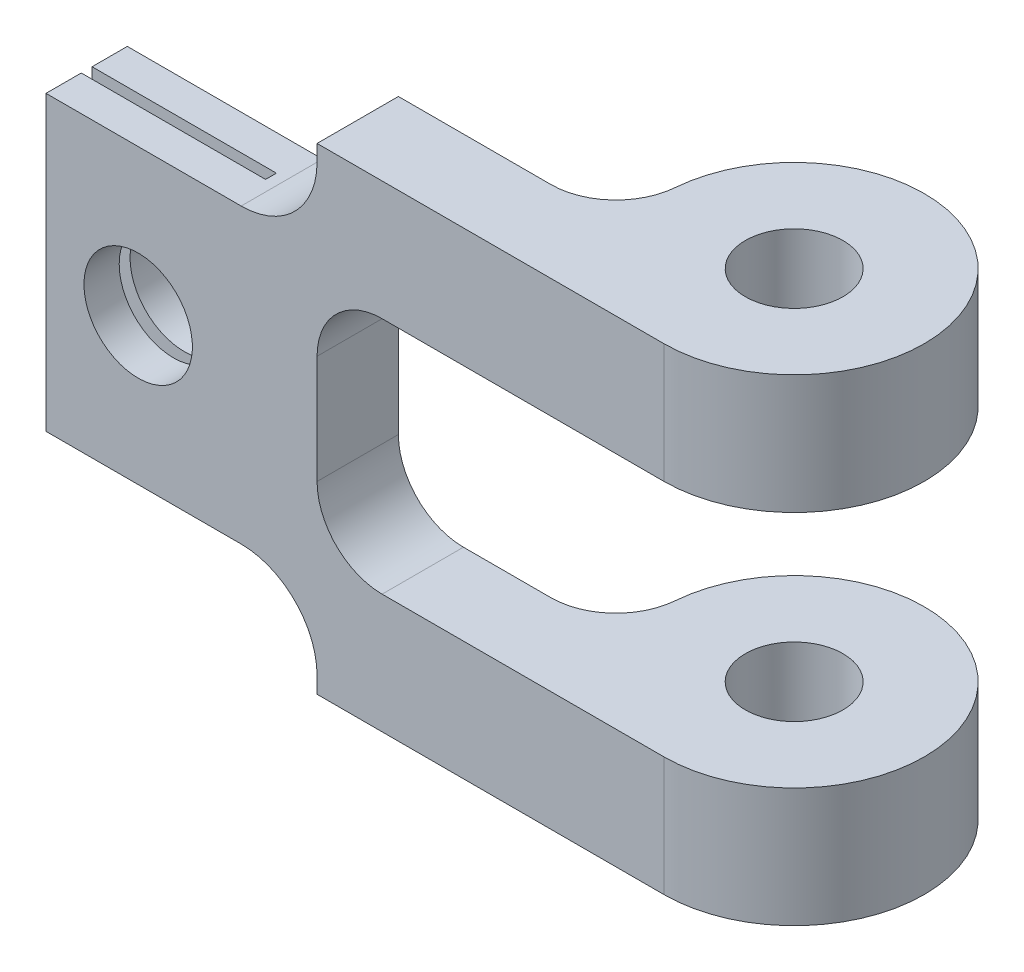
ISO-10303-21;
HEADER;
FILE_DESCRIPTION(('STEP AP214'),'2;1');
FILE_NAME('part.step','',(''),(''),'','','');
FILE_SCHEMA(('AUTOMOTIVE_DESIGN { 1 0 10303 214 1 1 1 1 }'));
ENDSEC;
DATA;
#1=APPLICATION_CONTEXT('core data for automotive mechanical design processes');
#2=APPLICATION_PROTOCOL_DEFINITION('international standard','automotive_design',2000,#1);
#3=PRODUCT_CONTEXT('',#1,'mechanical');
#4=PRODUCT('Part','Part','',(#3));
#5=PRODUCT_RELATED_PRODUCT_CATEGORY('part','',(#4));
#6=PRODUCT_DEFINITION_FORMATION('','',#4);
#7=PRODUCT_DEFINITION_CONTEXT('part definition',#1,'design');
#8=PRODUCT_DEFINITION('design','',#6,#7);
#9=PRODUCT_DEFINITION_SHAPE('','',#8);
#10=(LENGTH_UNIT() NAMED_UNIT(*) SI_UNIT(.MILLI.,.METRE.));
#11=(NAMED_UNIT(*) PLANE_ANGLE_UNIT() SI_UNIT($,.RADIAN.));
#12=(NAMED_UNIT(*) SI_UNIT($,.STERADIAN.) SOLID_ANGLE_UNIT());
#13=UNCERTAINTY_MEASURE_WITH_UNIT(LENGTH_MEASURE(1.E-05),#10,'distance_accuracy_value','');
#14=(GEOMETRIC_REPRESENTATION_CONTEXT(3) GLOBAL_UNCERTAINTY_ASSIGNED_CONTEXT((#13)) GLOBAL_UNIT_ASSIGNED_CONTEXT((#10,
#11,#12)) REPRESENTATION_CONTEXT('',''));
#15=CARTESIAN_POINT('',(0.,0.,0.));
#16=DIRECTION('',(0.,0.,1.));
#17=DIRECTION('',(1.,0.,0.));
#18=AXIS2_PLACEMENT_3D('',#15,#16,#17);
#19=CARTESIAN_POINT('',(-35.8747822293042,44.,-2.99999999999999));
#20=DIRECTION('',(0.,-1.,0.));
#21=DIRECTION('',(0.,0.,-1.));
#22=AXIS2_PLACEMENT_3D('',#19,#20,#21);
#23=CYLINDRICAL_SURFACE('',#22,12.);
#24=DIRECTION('',(0.,-1.,0.));
#25=VECTOR('',#24,1.);
#26=CARTESIAN_POINT('',(-23.9165214862028,44.,-1.99999999999999));
#27=LINE('',#26,#25);
#28=CARTESIAN_POINT('',(-23.9165214862028,44.,-1.99999999999999));
#29=VERTEX_POINT('',#28);
#30=CARTESIAN_POINT('',(-23.9165214862028,22.,-1.99999999999999));
#31=VERTEX_POINT('',#30);
#32=EDGE_CURVE('E437',#29,#31,#27,.T.);
#33=ORIENTED_EDGE('',*,*,#32,.T.);
#34=CARTESIAN_POINT('',(-35.8747822293042,22.,-2.99999999999999));
#35=DIRECTION('',(0.,1.,0.));
#36=DIRECTION('',(0.,0.,1.));
#37=AXIS2_PLACEMENT_3D('',#34,#35,#36);
#38=CIRCLE('',#37,12.);
#39=CARTESIAN_POINT('',(-35.8747822293042,22.,9.00000000000001));
#40=VERTEX_POINT('',#39);
#41=EDGE_CURVE('E290',#31,#40,#38,.F.);
#42=ORIENTED_EDGE('',*,*,#41,.T.);
#43=DIRECTION('',(0.,-1.,0.));
#44=VECTOR('',#43,1.);
#45=CARTESIAN_POINT('',(-35.8747822293042,44.,9.00000000000001));
#46=LINE('',#45,#44);
#47=CARTESIAN_POINT('',(-35.8747822293042,44.,9.00000000000001));
#48=VERTEX_POINT('',#47);
#49=EDGE_CURVE('E451',#48,#40,#46,.T.);
#50=ORIENTED_EDGE('',*,*,#49,.F.);
#51=CARTESIAN_POINT('',(-35.8747822293042,44.,-2.99999999999999));
#52=DIRECTION('',(0.,-1.,0.));
#53=DIRECTION('',(0.,0.,-1.));
#54=AXIS2_PLACEMENT_3D('',#51,#52,#53);
#55=CIRCLE('',#54,12.);
#56=EDGE_CURVE('E411',#29,#48,#55,.T.);
#57=ORIENTED_EDGE('',*,*,#56,.F.);
#58=EDGE_LOOP('',(#33,#42,#50,#57));
#59=FACE_BOUND('',#58,.T.);
#60=ADVANCED_FACE('F39',(#59),#23,.F.);
#61=CARTESIAN_POINT('',(0.,44.,0.));
#62=DIRECTION('',(0.,-1.,0.));
#63=DIRECTION('',(0.,0.,-1.));
#64=AXIS2_PLACEMENT_3D('',#61,#62,#63);
#65=CYLINDRICAL_SURFACE('',#64,24.);
#66=DIRECTION('',(0.,-1.,0.));
#67=VECTOR('',#66,1.);
#68=CARTESIAN_POINT('',(0.,44.,24.));
#69=LINE('',#68,#67);
#70=CARTESIAN_POINT('',(0.,44.,24.));
#71=VERTEX_POINT('',#70);
#72=CARTESIAN_POINT('',(0.,22.,24.));
#73=VERTEX_POINT('',#72);
#74=EDGE_CURVE('E442',#71,#73,#69,.T.);
#75=ORIENTED_EDGE('',*,*,#74,.T.);
#76=CARTESIAN_POINT('',(0.,22.,0.));
#77=DIRECTION('',(0.,1.,0.));
#78=DIRECTION('',(0.,0.,1.));
#79=AXIS2_PLACEMENT_3D('',#76,#77,#78);
#80=CIRCLE('',#79,24.);
#81=EDGE_CURVE('E284',#73,#31,#80,.T.);
#82=ORIENTED_EDGE('',*,*,#81,.T.);
#83=ORIENTED_EDGE('',*,*,#32,.F.);
#84=CARTESIAN_POINT('',(0.,44.,0.));
#85=DIRECTION('',(0.,1.,0.));
#86=DIRECTION('',(0.,0.,1.));
#87=AXIS2_PLACEMENT_3D('',#84,#85,#86);
#88=CIRCLE('',#87,24.);
#89=EDGE_CURVE('E421',#71,#29,#88,.T.);
#90=ORIENTED_EDGE('',*,*,#89,.F.);
#91=EDGE_LOOP('',(#75,#82,#83,#90));
#92=FACE_BOUND('',#91,.T.);
#93=ADVANCED_FACE('F509',(#92),#65,.T.);
#94=CARTESIAN_POINT('',(0.,44.,0.));
#95=DIRECTION('',(0.,-1.,0.));
#96=DIRECTION('',(0.,0.,-1.));
#97=AXIS2_PLACEMENT_3D('',#94,#95,#96);
#98=CYLINDRICAL_SURFACE('',#97,9.);
#99=CARTESIAN_POINT('',(0.,22.,0.));
#100=DIRECTION('',(0.,1.,0.));
#101=DIRECTION('',(0.,0.,1.));
#102=AXIS2_PLACEMENT_3D('',#99,#100,#101);
#103=CIRCLE('',#102,9.);
#104=CARTESIAN_POINT('',(0.,22.,9.));
#105=VERTEX_POINT('',#104);
#106=EDGE_CURVE('E43',#105,#105,#103,.T.);
#107=ORIENTED_EDGE('',*,*,#106,.F.);
#108=EDGE_LOOP('',(#107));
#109=FACE_BOUND('',#108,.T.);
#110=CARTESIAN_POINT('',(0.,44.,0.));
#111=DIRECTION('',(0.,1.,0.));
#112=DIRECTION('',(0.,0.,1.));
#113=AXIS2_PLACEMENT_3D('',#110,#111,#112);
#114=CIRCLE('',#113,9.);
#115=CARTESIAN_POINT('',(0.,44.,9.));
#116=VERTEX_POINT('',#115);
#117=EDGE_CURVE('E410',#116,#116,#114,.T.);
#118=ORIENTED_EDGE('',*,*,#117,.T.);
#119=EDGE_LOOP('',(#118));
#120=FACE_BOUND('',#119,.T.);
#121=ADVANCED_FACE('F486',(#109,#120),#98,.F.);
#122=CARTESIAN_POINT('',(-114.,44.001,17.5));
#123=DIRECTION('',(0.,0.,1.));
#124=DIRECTION('',(1.,0.,0.));
#125=AXIS2_PLACEMENT_3D('',#122,#123,#124);
#126=PLANE('',#125);
#127=DIRECTION('',(0.,-1.,0.));
#128=VECTOR('',#127,1.);
#129=CARTESIAN_POINT('',(-80.,44.001,17.5));
#130=LINE('',#129,#128);
#131=CARTESIAN_POINT('',(-80.,27.,17.5));
#132=VERTEX_POINT('',#131);
#133=CARTESIAN_POINT('',(-80.,20.3541019662497,17.5));
#134=VERTEX_POINT('',#133);
#135=EDGE_CURVE('E357',#132,#134,#130,.T.);
#136=ORIENTED_EDGE('',*,*,#135,.T.);
#137=DIRECTION('',(-1.,0.,0.));
#138=VECTOR('',#137,1.);
#139=CARTESIAN_POINT('',(-64.,20.3541019662497,17.5));
#140=LINE('',#139,#138);
#141=CARTESIAN_POINT('',(-114.,20.3541019662497,17.5));
#142=VERTEX_POINT('',#141);
#143=EDGE_CURVE('E329',#134,#142,#140,.T.);
#144=ORIENTED_EDGE('',*,*,#143,.T.);
#145=DIRECTION('',(0.,-1.,0.));
#146=VECTOR('',#145,1.);
#147=CARTESIAN_POINT('',(-114.,44.001,17.5));
#148=LINE('',#147,#146);
#149=CARTESIAN_POINT('',(-114.,27.,17.5));
#150=VERTEX_POINT('',#149);
#151=EDGE_CURVE('E352',#150,#142,#148,.T.);
#152=ORIENTED_EDGE('',*,*,#151,.F.);
#153=DIRECTION('',(-1.,0.,0.));
#154=VECTOR('',#153,1.);
#155=CARTESIAN_POINT('',(-114.,27.,17.5));
#156=LINE('',#155,#154);
#157=EDGE_CURVE('E343',#132,#150,#156,.T.);
#158=ORIENTED_EDGE('',*,*,#157,.F.);
#159=EDGE_LOOP('',(#136,#144,#152,#158));
#160=FACE_BOUND('',#159,.T.);
#161=ADVANCED_FACE('F605',(#160),#126,.F.);
#162=CARTESIAN_POINT('',(-97.,0.,17.5));
#163=DIRECTION('',(0.,0.,1.));
#164=DIRECTION('',(1.,0.,0.));
#165=AXIS2_PLACEMENT_3D('',#162,#163,#164);
#166=CIRCLE('',#165,9.99999999999999);
#167=CARTESIAN_POINT('',(-87.,0.,17.5));
#168=VERTEX_POINT('',#167);
#169=EDGE_CURVE('E331',#168,#168,#166,.T.);
#170=ORIENTED_EDGE('',*,*,#169,.T.);
#171=EDGE_LOOP('',(#170));
#172=FACE_BOUND('',#171,.T.);
#173=CARTESIAN_POINT('',(-114.,13.6458980337503,17.5));
#174=VERTEX_POINT('',#173);
#175=CARTESIAN_POINT('',(-114.,-13.6458980337503,17.5));
#176=VERTEX_POINT('',#175);
#177=EDGE_CURVE('E356',#174,#176,#148,.T.);
#178=ORIENTED_EDGE('',*,*,#177,.F.);
#179=DIRECTION('',(-1.,0.,0.));
#180=VECTOR('',#179,1.);
#181=CARTESIAN_POINT('',(-64.,13.6458980337503,17.5));
#182=LINE('',#181,#180);
#183=CARTESIAN_POINT('',(-80.,13.6458980337503,17.5));
#184=VERTEX_POINT('',#183);
#185=EDGE_CURVE('E322',#174,#184,#182,.F.);
#186=ORIENTED_EDGE('',*,*,#185,.T.);
#187=CARTESIAN_POINT('',(-80.,-13.6458980337503,17.5));
#188=VERTEX_POINT('',#187);
#189=EDGE_CURVE('E361',#184,#188,#130,.T.);
#190=ORIENTED_EDGE('',*,*,#189,.T.);
#191=DIRECTION('',(-1.,0.,0.));
#192=VECTOR('',#191,1.);
#193=CARTESIAN_POINT('',(-64.,-13.6458980337503,17.5));
#194=LINE('',#193,#192);
#195=EDGE_CURVE('E319',#188,#176,#194,.T.);
#196=ORIENTED_EDGE('',*,*,#195,.T.);
#197=EDGE_LOOP('',(#178,#186,#190,#196));
#198=FACE_BOUND('',#197,.T.);
#199=ADVANCED_FACE('F610',(#172,#198),#126,.F.);
#200=CARTESIAN_POINT('',(-114.,44.001,15.5));
#201=DIRECTION('',(0.,0.,-1.));
#202=DIRECTION('',(-1.,0.,0.));
#203=AXIS2_PLACEMENT_3D('',#200,#201,#202);
#204=PLANE('',#203);
#205=CARTESIAN_POINT('',(-97.,0.,15.5));
#206=DIRECTION('',(0.,0.,-1.));
#207=DIRECTION('',(-1.,0.,0.));
#208=AXIS2_PLACEMENT_3D('',#205,#206,#207);
#209=CIRCLE('',#208,9.99999999999999);
#210=CARTESIAN_POINT('',(-107.,0.,15.5));
#211=VERTEX_POINT('',#210);
#212=EDGE_CURVE('E360',#211,#211,#209,.T.);
#213=ORIENTED_EDGE('',*,*,#212,.T.);
#214=EDGE_LOOP('',(#213));
#215=FACE_BOUND('',#214,.T.);
#216=DIRECTION('',(0.,-1.,0.));
#217=VECTOR('',#216,1.);
#218=CARTESIAN_POINT('',(-80.,44.001,15.5));
#219=LINE('',#218,#217);
#220=CARTESIAN_POINT('',(-80.,13.6458980337503,15.5));
#221=VERTEX_POINT('',#220);
#222=CARTESIAN_POINT('',(-80.,-13.6458980337503,15.5));
#223=VERTEX_POINT('',#222);
#224=EDGE_CURVE('E366',#221,#223,#219,.T.);
#225=ORIENTED_EDGE('',*,*,#224,.F.);
#226=DIRECTION('',(-1.,0.,0.));
#227=VECTOR('',#226,1.);
#228=CARTESIAN_POINT('',(-64.,13.6458980337503,15.5));
#229=LINE('',#228,#227);
#230=CARTESIAN_POINT('',(-114.,13.6458980337503,15.5));
#231=VERTEX_POINT('',#230);
#232=EDGE_CURVE('E62',#221,#231,#229,.T.);
#233=ORIENTED_EDGE('',*,*,#232,.T.);
#234=DIRECTION('',(0.,-1.,0.));
#235=VECTOR('',#234,1.);
#236=CARTESIAN_POINT('',(-114.,44.001,15.5));
#237=LINE('',#236,#235);
#238=CARTESIAN_POINT('',(-114.,-13.6458980337503,15.5));
#239=VERTEX_POINT('',#238);
#240=EDGE_CURVE('E373',#231,#239,#237,.T.);
#241=ORIENTED_EDGE('',*,*,#240,.T.);
#242=DIRECTION('',(-1.,0.,0.));
#243=VECTOR('',#242,1.);
#244=CARTESIAN_POINT('',(-64.,-13.6458980337503,15.5));
#245=LINE('',#244,#243);
#246=EDGE_CURVE('E320',#239,#223,#245,.F.);
#247=ORIENTED_EDGE('',*,*,#246,.T.);
#248=EDGE_LOOP('',(#225,#233,#241,#247));
#249=FACE_BOUND('',#248,.T.);
#250=ADVANCED_FACE('F633',(#215,#249),#204,.F.);
#251=CARTESIAN_POINT('',(-80.,-20.3541019662497,15.5));
#252=VERTEX_POINT('',#251);
#253=CARTESIAN_POINT('',(-80.,-27.,15.5));
#254=VERTEX_POINT('',#253);
#255=EDGE_CURVE('E369',#252,#254,#219,.T.);
#256=ORIENTED_EDGE('',*,*,#255,.F.);
#257=DIRECTION('',(-1.,0.,0.));
#258=VECTOR('',#257,1.);
#259=CARTESIAN_POINT('',(-64.,-20.3541019662497,15.5));
#260=LINE('',#259,#258);
#261=CARTESIAN_POINT('',(-114.,-20.3541019662497,15.5));
#262=VERTEX_POINT('',#261);
#263=EDGE_CURVE('E57',#252,#262,#260,.T.);
#264=ORIENTED_EDGE('',*,*,#263,.T.);
#265=CARTESIAN_POINT('',(-114.,-27.,15.5));
#266=VERTEX_POINT('',#265);
#267=EDGE_CURVE('E351',#262,#266,#237,.T.);
#268=ORIENTED_EDGE('',*,*,#267,.T.);
#269=DIRECTION('',(1.,0.,0.));
#270=VECTOR('',#269,1.);
#271=CARTESIAN_POINT('',(-114.,-27.,15.5));
#272=LINE('',#271,#270);
#273=EDGE_CURVE('E344',#266,#254,#272,.T.);
#274=ORIENTED_EDGE('',*,*,#273,.T.);
#275=EDGE_LOOP('',(#256,#264,#268,#274));
#276=FACE_BOUND('',#275,.T.);
#277=ADVANCED_FACE('F619',(#276),#204,.F.);
#278=CARTESIAN_POINT('',(-80.,44.001,17.5));
#279=DIRECTION('',(1.,0.,0.));
#280=DIRECTION('',(0.,0.,-1.));
#281=AXIS2_PLACEMENT_3D('',#278,#279,#280);
#282=PLANE('',#281);
#283=CARTESIAN_POINT('',(-80.,27.,15.5));
#284=VERTEX_POINT('',#283);
#285=CARTESIAN_POINT('',(-80.,20.3541019662497,15.5));
#286=VERTEX_POINT('',#285);
#287=EDGE_CURVE('E364',#284,#286,#219,.T.);
#288=ORIENTED_EDGE('',*,*,#287,.T.);
#289=CARTESIAN_POINT('',(-80.,17.,16.5));
#290=DIRECTION('',(1.,0.,0.));
#291=DIRECTION('',(0.,0.,-1.));
#292=AXIS2_PLACEMENT_3D('',#289,#290,#291);
#293=CIRCLE('',#292,3.5);
#294=EDGE_CURVE('E11',#286,#134,#293,.T.);
#295=ORIENTED_EDGE('',*,*,#294,.T.);
#296=ORIENTED_EDGE('',*,*,#135,.F.);
#297=DIRECTION('',(0.,0.,1.));
#298=VECTOR('',#297,1.);
#299=CARTESIAN_POINT('',(-80.,27.,17.5));
#300=LINE('',#299,#298);
#301=EDGE_CURVE('E334',#284,#132,#300,.T.);
#302=ORIENTED_EDGE('',*,*,#301,.F.);
#303=EDGE_LOOP('',(#288,#295,#296,#302));
#304=FACE_BOUND('',#303,.T.);
#305=ADVANCED_FACE('F535',(#304),#282,.F.);
#306=ORIENTED_EDGE('',*,*,#189,.F.);
#307=EDGE_CURVE('E48',#184,#221,#293,.T.);
#308=ORIENTED_EDGE('',*,*,#307,.T.);
#309=ORIENTED_EDGE('',*,*,#224,.T.);
#310=CARTESIAN_POINT('',(-80.,-17.,16.5));
#311=DIRECTION('',(1.,0.,0.));
#312=DIRECTION('',(0.,0.,-1.));
#313=AXIS2_PLACEMENT_3D('',#310,#311,#312);
#314=CIRCLE('',#313,3.5);
#315=EDGE_CURVE('E474',#223,#188,#314,.T.);
#316=ORIENTED_EDGE('',*,*,#315,.T.);
#317=EDGE_LOOP('',(#306,#308,#309,#316));
#318=FACE_BOUND('',#317,.T.);
#319=ADVANCED_FACE('F531',(#318),#282,.F.);
#320=CARTESIAN_POINT('',(-114.,27.,97.5934779718964));
#321=DIRECTION('',(-1.,0.,0.));
#322=DIRECTION('',(0.,0.,1.));
#323=AXIS2_PLACEMENT_3D('',#320,#321,#322);
#324=PLANE('',#323);
#325=CARTESIAN_POINT('',(-114.,17.,16.5));
#326=DIRECTION('',(-1.,0.,0.));
#327=DIRECTION('',(0.,0.,1.));
#328=AXIS2_PLACEMENT_3D('',#325,#326,#327);
#329=CIRCLE('',#328,3.5);
#330=EDGE_CURVE('E308',#174,#142,#329,.T.);
#331=ORIENTED_EDGE('',*,*,#330,.F.);
#332=ORIENTED_EDGE('',*,*,#177,.T.);
#333=CARTESIAN_POINT('',(-114.,-17.,16.5));
#334=DIRECTION('',(-1.,0.,0.));
#335=DIRECTION('',(0.,0.,-1.));
#336=AXIS2_PLACEMENT_3D('',#333,#334,#335);
#337=CIRCLE('',#336,3.5);
#338=CARTESIAN_POINT('',(-114.,-20.3541019662497,17.5));
#339=VERTEX_POINT('',#338);
#340=EDGE_CURVE('E313',#339,#176,#337,.T.);
#341=ORIENTED_EDGE('',*,*,#340,.F.);
#342=CARTESIAN_POINT('',(-114.,-27.,17.5));
#343=VERTEX_POINT('',#342);
#344=EDGE_CURVE('E359',#339,#343,#148,.T.);
#345=ORIENTED_EDGE('',*,*,#344,.T.);
#346=DIRECTION('',(0.,0.,-1.));
#347=VECTOR('',#346,1.);
#348=CARTESIAN_POINT('',(-114.,-27.,97.5934779718964));
#349=LINE('',#348,#347);
#350=CARTESIAN_POINT('',(-114.,-27.,24.));
#351=VERTEX_POINT('',#350);
#352=EDGE_CURVE('E402',#351,#343,#349,.T.);
#353=ORIENTED_EDGE('',*,*,#352,.F.);
#354=DIRECTION('',(0.,-1.,0.));
#355=VECTOR('',#354,1.);
#356=CARTESIAN_POINT('',(-114.,27.,24.));
#357=LINE('',#356,#355);
#358=CARTESIAN_POINT('',(-114.,27.,24.));
#359=VERTEX_POINT('',#358);
#360=EDGE_CURVE('E383',#359,#351,#357,.T.);
#361=ORIENTED_EDGE('',*,*,#360,.F.);
#362=DIRECTION('',(0.,0.,-1.));
#363=VECTOR('',#362,1.);
#364=CARTESIAN_POINT('',(-114.,27.,97.5934779718964));
#365=LINE('',#364,#363);
#366=EDGE_CURVE('E390',#359,#150,#365,.T.);
#367=ORIENTED_EDGE('',*,*,#366,.T.);
#368=ORIENTED_EDGE('',*,*,#151,.T.);
#369=EDGE_LOOP('',(#331,#332,#341,#345,#353,#361,#367,#368));
#370=FACE_BOUND('',#369,.T.);
#371=ADVANCED_FACE('F579',(#370),#324,.T.);
#372=CARTESIAN_POINT('',(-97.,0.,24.001));
#373=DIRECTION('',(0.,0.,-1.));
#374=DIRECTION('',(-1.,0.,0.));
#375=AXIS2_PLACEMENT_3D('',#372,#373,#374);
#376=CYLINDRICAL_SURFACE('',#375,9.99999999999999);
#377=ORIENTED_EDGE('',*,*,#169,.F.);
#378=EDGE_LOOP('',(#377));
#379=FACE_BOUND('',#378,.T.);
#380=CARTESIAN_POINT('',(-97.,0.,24.));
#381=DIRECTION('',(0.,0.,-1.));
#382=DIRECTION('',(-1.,0.,0.));
#383=AXIS2_PLACEMENT_3D('',#380,#381,#382);
#384=CIRCLE('',#383,9.99999999999999);
#385=CARTESIAN_POINT('',(-107.,0.,24.));
#386=VERTEX_POINT('',#385);
#387=EDGE_CURVE('E379',#386,#386,#384,.F.);
#388=ORIENTED_EDGE('',*,*,#387,.T.);
#389=EDGE_LOOP('',(#388));
#390=FACE_BOUND('',#389,.T.);
#391=ADVANCED_FACE('F632',(#379,#390),#376,.F.);
#392=CARTESIAN_POINT('',(-64.,44.,24.));
#393=DIRECTION('',(1.,0.,0.));
#394=DIRECTION('',(0.,0.,-1.));
#395=AXIS2_PLACEMENT_3D('',#392,#393,#394);
#396=PLANE('',#395);
#397=DIRECTION('',(0.,-1.,0.));
#398=VECTOR('',#397,1.);
#399=CARTESIAN_POINT('',(-64.,44.,9.00000000000001));
#400=LINE('',#399,#398);
#401=CARTESIAN_POINT('',(-64.,44.,9.00000000000001));
#402=VERTEX_POINT('',#401);
#403=CARTESIAN_POINT('',(-64.,41.,9.00000000000001));
#404=VERTEX_POINT('',#403);
#405=EDGE_CURVE('E447',#402,#404,#400,.T.);
#406=ORIENTED_EDGE('',*,*,#405,.T.);
#407=DIRECTION('',(0.,0.,-1.));
#408=VECTOR('',#407,1.);
#409=CARTESIAN_POINT('',(-64.,41.,24.));
#410=LINE('',#409,#408);
#411=CARTESIAN_POINT('',(-64.,41.,24.));
#412=VERTEX_POINT('',#411);
#413=EDGE_CURVE('E462',#404,#412,#410,.F.);
#414=ORIENTED_EDGE('',*,*,#413,.T.);
#415=DIRECTION('',(0.,-1.,0.));
#416=VECTOR('',#415,1.);
#417=CARTESIAN_POINT('',(-64.,44.,24.));
#418=LINE('',#417,#416);
#419=CARTESIAN_POINT('',(-64.,44.,24.));
#420=VERTEX_POINT('',#419);
#421=EDGE_CURVE('E443',#420,#412,#418,.T.);
#422=ORIENTED_EDGE('',*,*,#421,.F.);
#423=DIRECTION('',(0.,0.,1.));
#424=VECTOR('',#423,1.);
#425=CARTESIAN_POINT('',(-64.,44.,24.));
#426=LINE('',#425,#424);
#427=EDGE_CURVE('E420',#402,#420,#426,.T.);
#428=ORIENTED_EDGE('',*,*,#427,.F.);
#429=EDGE_LOOP('',(#406,#414,#422,#428));
#430=FACE_BOUND('',#429,.T.);
#431=ADVANCED_FACE('F501',(#430),#396,.F.);
#432=CARTESIAN_POINT('',(-35.8747822293042,44.,-2.99999999999999));
#433=DIRECTION('',(0.,-1.,0.));
#434=DIRECTION('',(0.,0.,-1.));
#435=AXIS2_PLACEMENT_3D('',#432,#433,#434);
#436=PLANE('',#435);
#437=ORIENTED_EDGE('',*,*,#56,.T.);
#438=DIRECTION('',(-1.,0.,0.));
#439=VECTOR('',#438,1.);
#440=CARTESIAN_POINT('',(-35.8747822293042,44.,9.00000000000001));
#441=LINE('',#440,#439);
#442=EDGE_CURVE('E418',#48,#402,#441,.T.);
#443=ORIENTED_EDGE('',*,*,#442,.T.);
#444=ORIENTED_EDGE('',*,*,#427,.T.);
#445=DIRECTION('',(1.,0.,0.));
#446=VECTOR('',#445,1.);
#447=CARTESIAN_POINT('',(0.,44.,24.));
#448=LINE('',#447,#446);
#449=EDGE_CURVE('E423',#420,#71,#448,.T.);
#450=ORIENTED_EDGE('',*,*,#449,.T.);
#451=ORIENTED_EDGE('',*,*,#89,.T.);
#452=EDGE_LOOP('',(#437,#443,#444,#450,#451));
#453=FACE_BOUND('',#452,.T.);
#454=ORIENTED_EDGE('',*,*,#117,.F.);
#455=EDGE_LOOP('',(#454));
#456=FACE_BOUND('',#455,.T.);
#457=ADVANCED_FACE('F495',(#453,#456),#436,.F.);
#458=CARTESIAN_POINT('',(-35.8747822293042,-44.,-2.99999999999999));
#459=DIRECTION('',(0.,-1.,0.));
#460=DIRECTION('',(0.,0.,-1.));
#461=AXIS2_PLACEMENT_3D('',#458,#459,#460);
#462=PLANE('',#461);
#463=CARTESIAN_POINT('',(-35.8747822293042,-44.,-2.99999999999999));
#464=DIRECTION('',(0.,-1.,0.));
#465=DIRECTION('',(0.,0.,-1.));
#466=AXIS2_PLACEMENT_3D('',#463,#464,#465);
#467=CIRCLE('',#466,12.);
#468=CARTESIAN_POINT('',(-23.9165214862028,-44.,-1.99999999999999));
#469=VERTEX_POINT('',#468);
#470=CARTESIAN_POINT('',(-35.8747822293042,-44.,9.00000000000001));
#471=VERTEX_POINT('',#470);
#472=EDGE_CURVE('E409',#469,#471,#467,.T.);
#473=ORIENTED_EDGE('',*,*,#472,.F.);
#474=CARTESIAN_POINT('',(0.,-44.,0.));
#475=DIRECTION('',(0.,1.,0.));
#476=DIRECTION('',(0.,0.,1.));
#477=AXIS2_PLACEMENT_3D('',#474,#475,#476);
#478=CIRCLE('',#477,24.);
#479=CARTESIAN_POINT('',(0.,-44.,24.));
#480=VERTEX_POINT('',#479);
#481=EDGE_CURVE('E417',#480,#469,#478,.T.);
#482=ORIENTED_EDGE('',*,*,#481,.F.);
#483=DIRECTION('',(1.,0.,0.));
#484=VECTOR('',#483,1.);
#485=CARTESIAN_POINT('',(0.,-44.,24.));
#486=LINE('',#485,#484);
#487=CARTESIAN_POINT('',(-64.,-44.,24.));
#488=VERTEX_POINT('',#487);
#489=EDGE_CURVE('E432',#488,#480,#486,.T.);
#490=ORIENTED_EDGE('',*,*,#489,.F.);
#491=DIRECTION('',(0.,0.,1.));
#492=VECTOR('',#491,1.);
#493=CARTESIAN_POINT('',(-64.,-44.,24.));
#494=LINE('',#493,#492);
#495=CARTESIAN_POINT('',(-64.,-44.,9.00000000000001));
#496=VERTEX_POINT('',#495);
#497=EDGE_CURVE('E431',#496,#488,#494,.T.);
#498=ORIENTED_EDGE('',*,*,#497,.F.);
#499=DIRECTION('',(-1.,0.,0.));
#500=VECTOR('',#499,1.);
#501=CARTESIAN_POINT('',(-35.8747822293042,-44.,9.00000000000001));
#502=LINE('',#501,#500);
#503=EDGE_CURVE('E428',#471,#496,#502,.T.);
#504=ORIENTED_EDGE('',*,*,#503,.F.);
#505=EDGE_LOOP('',(#473,#482,#490,#498,#504));
#506=FACE_BOUND('',#505,.T.);
#507=CARTESIAN_POINT('',(0.,-44.,0.));
#508=DIRECTION('',(0.,1.,0.));
#509=DIRECTION('',(0.,0.,1.));
#510=AXIS2_PLACEMENT_3D('',#507,#508,#509);
#511=CIRCLE('',#510,9.);
#512=CARTESIAN_POINT('',(0.,-44.,9.));
#513=VERTEX_POINT('',#512);
#514=EDGE_CURVE('E408',#513,#513,#511,.T.);
#515=ORIENTED_EDGE('',*,*,#514,.T.);
#516=EDGE_LOOP('',(#515));
#517=FACE_BOUND('',#516,.T.);
#518=ADVANCED_FACE('F487',(#506,#517),#462,.T.);
#519=CARTESIAN_POINT('',(-35.8747822293042,-22.,9.00000000000001));
#520=VERTEX_POINT('',#519);
#521=EDGE_CURVE('E455',#520,#471,#46,.T.);
#522=ORIENTED_EDGE('',*,*,#521,.F.);
#523=CARTESIAN_POINT('',(-35.8747822293042,-22.,-2.99999999999999));
#524=DIRECTION('',(0.,-1.,0.));
#525=DIRECTION('',(0.,0.,-1.));
#526=AXIS2_PLACEMENT_3D('',#523,#524,#525);
#527=CIRCLE('',#526,12.);
#528=CARTESIAN_POINT('',(-23.9165214862028,-22.,-1.99999999999999));
#529=VERTEX_POINT('',#528);
#530=EDGE_CURVE('E283',#520,#529,#527,.F.);
#531=ORIENTED_EDGE('',*,*,#530,.T.);
#532=EDGE_CURVE('E422',#529,#469,#27,.T.);
#533=ORIENTED_EDGE('',*,*,#532,.T.);
#534=ORIENTED_EDGE('',*,*,#472,.T.);
#535=EDGE_LOOP('',(#522,#531,#533,#534));
#536=FACE_BOUND('',#535,.T.);
#537=ADVANCED_FACE('F491',(#536),#23,.F.);
#538=CARTESIAN_POINT('',(-35.8747822293042,44.,9.00000000000001));
#539=DIRECTION('',(0.,0.,1.));
#540=DIRECTION('',(1.,0.,0.));
#541=AXIS2_PLACEMENT_3D('',#538,#539,#540);
#542=PLANE('',#541);
#543=CARTESIAN_POINT('',(-97.,0.,9.00000000000001));
#544=DIRECTION('',(0.,0.,-1.));
#545=DIRECTION('',(-1.,0.,0.));
#546=AXIS2_PLACEMENT_3D('',#543,#544,#545);
#547=CIRCLE('',#546,9.99999999999999);
#548=CARTESIAN_POINT('',(-107.,0.,9.00000000000001));
#549=VERTEX_POINT('',#548);
#550=EDGE_CURVE('E340',#549,#549,#547,.T.);
#551=ORIENTED_EDGE('',*,*,#550,.F.);
#552=EDGE_LOOP('',(#551));
#553=FACE_BOUND('',#552,.T.);
#554=ORIENTED_EDGE('',*,*,#49,.T.);
#555=DIRECTION('',(-1.,0.,0.));
#556=VECTOR('',#555,1.);
#557=CARTESIAN_POINT('',(-35.8747822293042,22.,9.00000000000001));
#558=LINE('',#557,#556);
#559=CARTESIAN_POINT('',(-51.9999999999999,22.,9.00000000000001));
#560=VERTEX_POINT('',#559);
#561=EDGE_CURVE('E287',#40,#560,#558,.T.);
#562=ORIENTED_EDGE('',*,*,#561,.T.);
#563=CARTESIAN_POINT('',(-52.,10.,9.00000000000001));
#564=DIRECTION('',(0.,0.,1.));
#565=DIRECTION('',(1.,0.,0.));
#566=AXIS2_PLACEMENT_3D('',#563,#564,#565);
#567=CIRCLE('',#566,12.);
#568=CARTESIAN_POINT('',(-64.,9.99999999999992,9.00000000000001));
#569=VERTEX_POINT('',#568);
#570=EDGE_CURVE('E296',#560,#569,#567,.T.);
#571=ORIENTED_EDGE('',*,*,#570,.T.);
#572=DIRECTION('',(0.,-1.,0.));
#573=VECTOR('',#572,1.);
#574=CARTESIAN_POINT('',(-64.,44.,9.00000000000001));
#575=LINE('',#574,#573);
#576=CARTESIAN_POINT('',(-64.,-9.99999999999991,9.00000000000001));
#577=VERTEX_POINT('',#576);
#578=EDGE_CURVE('E293',#569,#577,#575,.T.);
#579=ORIENTED_EDGE('',*,*,#578,.T.);
#580=CARTESIAN_POINT('',(-52.,-10.,9.00000000000001));
#581=DIRECTION('',(0.,0.,1.));
#582=DIRECTION('',(1.,0.,0.));
#583=AXIS2_PLACEMENT_3D('',#580,#581,#582);
#584=CIRCLE('',#583,12.);
#585=CARTESIAN_POINT('',(-51.9999999999999,-22.,9.00000000000001));
#586=VERTEX_POINT('',#585);
#587=EDGE_CURVE('E291',#577,#586,#584,.T.);
#588=ORIENTED_EDGE('',*,*,#587,.T.);
#589=DIRECTION('',(1.,0.,0.));
#590=VECTOR('',#589,1.);
#591=CARTESIAN_POINT('',(-35.8747822293042,-22.,9.00000000000001));
#592=LINE('',#591,#590);
#593=EDGE_CURVE('E244',#586,#520,#592,.T.);
#594=ORIENTED_EDGE('',*,*,#593,.T.);
#595=ORIENTED_EDGE('',*,*,#521,.T.);
#596=ORIENTED_EDGE('',*,*,#503,.T.);
#597=CARTESIAN_POINT('',(-64.,-41.,9.00000000000001));
#598=VERTEX_POINT('',#597);
#599=EDGE_CURVE('E446',#598,#496,#400,.T.);
#600=ORIENTED_EDGE('',*,*,#599,.F.);
#601=CARTESIAN_POINT('',(-78.,-41.,9.00000000000001));
#602=DIRECTION('',(0.,0.,1.));
#603=DIRECTION('',(1.,0.,0.));
#604=AXIS2_PLACEMENT_3D('',#601,#602,#603);
#605=CIRCLE('',#604,14.);
#606=CARTESIAN_POINT('',(-78.,-27.,9.00000000000001));
#607=VERTEX_POINT('',#606);
#608=EDGE_CURVE('E468',#598,#607,#605,.T.);
#609=ORIENTED_EDGE('',*,*,#608,.T.);
#610=DIRECTION('',(-1.,0.,0.));
#611=VECTOR('',#610,1.);
#612=CARTESIAN_POINT('',(-64.,-27.,9.00000000000001));
#613=LINE('',#612,#611);
#614=CARTESIAN_POINT('',(-114.,-27.,9.00000000000001));
#615=VERTEX_POINT('',#614);
#616=EDGE_CURVE('E382',#607,#615,#613,.T.);
#617=ORIENTED_EDGE('',*,*,#616,.T.);
#618=DIRECTION('',(0.,1.,0.));
#619=VECTOR('',#618,1.);
#620=CARTESIAN_POINT('',(-114.,27.,9.00000000000001));
#621=LINE('',#620,#619);
#622=CARTESIAN_POINT('',(-114.,27.,9.00000000000001));
#623=VERTEX_POINT('',#622);
#624=EDGE_CURVE('E393',#615,#623,#621,.T.);
#625=ORIENTED_EDGE('',*,*,#624,.T.);
#626=DIRECTION('',(1.,0.,0.));
#627=VECTOR('',#626,1.);
#628=CARTESIAN_POINT('',(-64.,27.,9.00000000000001));
#629=LINE('',#628,#627);
#630=CARTESIAN_POINT('',(-78.,27.,9.00000000000001));
#631=VERTEX_POINT('',#630);
#632=EDGE_CURVE('E392',#623,#631,#629,.T.);
#633=ORIENTED_EDGE('',*,*,#632,.T.);
#634=CARTESIAN_POINT('',(-78.,41.,9.00000000000001));
#635=DIRECTION('',(0.,0.,1.));
#636=DIRECTION('',(1.,0.,0.));
#637=AXIS2_PLACEMENT_3D('',#634,#635,#636);
#638=CIRCLE('',#637,14.);
#639=EDGE_CURVE('E467',#631,#404,#638,.T.);
#640=ORIENTED_EDGE('',*,*,#639,.T.);
#641=ORIENTED_EDGE('',*,*,#405,.F.);
#642=ORIENTED_EDGE('',*,*,#442,.F.);
#643=EDGE_LOOP('',(#554,#562,#571,#579,#588,#594,#595,#596,#600,#609,#617,#625,#633,#640,#641,#642));
#644=FACE_BOUND('',#643,.T.);
#645=ADVANCED_FACE('F498',(#553,#644),#542,.F.);
#646=CARTESIAN_POINT('',(-64.,-41.,24.));
#647=VERTEX_POINT('',#646);
#648=EDGE_CURVE('E441',#647,#488,#418,.T.);
#649=ORIENTED_EDGE('',*,*,#648,.F.);
#650=DIRECTION('',(0.,0.,-1.));
#651=VECTOR('',#650,1.);
#652=CARTESIAN_POINT('',(-64.,-41.,24.));
#653=LINE('',#652,#651);
#654=EDGE_CURVE('E457',#647,#598,#653,.T.);
#655=ORIENTED_EDGE('',*,*,#654,.T.);
#656=ORIENTED_EDGE('',*,*,#599,.T.);
#657=ORIENTED_EDGE('',*,*,#497,.T.);
#658=EDGE_LOOP('',(#649,#655,#656,#657));
#659=FACE_BOUND('',#658,.T.);
#660=ADVANCED_FACE('F539',(#659),#396,.F.);
#661=CARTESIAN_POINT('',(0.,44.,24.));
#662=DIRECTION('',(0.,0.,-1.));
#663=DIRECTION('',(-1.,0.,0.));
#664=AXIS2_PLACEMENT_3D('',#661,#662,#663);
#665=PLANE('',#664);
#666=ORIENTED_EDGE('',*,*,#387,.F.);
#667=EDGE_LOOP('',(#666));
#668=FACE_BOUND('',#667,.T.);
#669=CARTESIAN_POINT('',(-52.,10.,24.));
#670=DIRECTION('',(0.,0.,-1.));
#671=DIRECTION('',(1.,0.,0.));
#672=AXIS2_PLACEMENT_3D('',#669,#670,#671);
#673=CIRCLE('',#672,12.);
#674=CARTESIAN_POINT('',(-64.,9.99999999999992,24.));
#675=VERTEX_POINT('',#674);
#676=CARTESIAN_POINT('',(-51.9999999999999,22.,24.));
#677=VERTEX_POINT('',#676);
#678=EDGE_CURVE('E270',#675,#677,#673,.T.);
#679=ORIENTED_EDGE('',*,*,#678,.T.);
#680=DIRECTION('',(1.,0.,0.));
#681=VECTOR('',#680,1.);
#682=CARTESIAN_POINT('',(24.,22.,24.));
#683=LINE('',#682,#681);
#684=EDGE_CURVE('E249',#677,#73,#683,.T.);
#685=ORIENTED_EDGE('',*,*,#684,.T.);
#686=ORIENTED_EDGE('',*,*,#74,.F.);
#687=ORIENTED_EDGE('',*,*,#449,.F.);
#688=ORIENTED_EDGE('',*,*,#421,.T.);
#689=CARTESIAN_POINT('',(-78.,41.,24.));
#690=DIRECTION('',(0.,0.,-1.));
#691=DIRECTION('',(-1.,0.,0.));
#692=AXIS2_PLACEMENT_3D('',#689,#690,#691);
#693=CIRCLE('',#692,14.);
#694=CARTESIAN_POINT('',(-78.,27.,24.));
#695=VERTEX_POINT('',#694);
#696=EDGE_CURVE('E472',#412,#695,#693,.T.);
#697=ORIENTED_EDGE('',*,*,#696,.T.);
#698=DIRECTION('',(-1.,0.,0.));
#699=VECTOR('',#698,1.);
#700=CARTESIAN_POINT('',(-64.,27.,24.));
#701=LINE('',#700,#699);
#702=EDGE_CURVE('E387',#695,#359,#701,.T.);
#703=ORIENTED_EDGE('',*,*,#702,.T.);
#704=ORIENTED_EDGE('',*,*,#360,.T.);
#705=DIRECTION('',(1.,0.,0.));
#706=VECTOR('',#705,1.);
#707=CARTESIAN_POINT('',(-64.,-27.,24.));
#708=LINE('',#707,#706);
#709=CARTESIAN_POINT('',(-78.,-27.,24.));
#710=VERTEX_POINT('',#709);
#711=EDGE_CURVE('E386',#351,#710,#708,.T.);
#712=ORIENTED_EDGE('',*,*,#711,.T.);
#713=CARTESIAN_POINT('',(-78.,-41.,24.));
#714=DIRECTION('',(0.,0.,-1.));
#715=DIRECTION('',(-1.,0.,0.));
#716=AXIS2_PLACEMENT_3D('',#713,#714,#715);
#717=CIRCLE('',#716,14.);
#718=EDGE_CURVE('E466',#710,#647,#717,.T.);
#719=ORIENTED_EDGE('',*,*,#718,.T.);
#720=ORIENTED_EDGE('',*,*,#648,.T.);
#721=ORIENTED_EDGE('',*,*,#489,.T.);
#722=CARTESIAN_POINT('',(0.,-22.,24.));
#723=VERTEX_POINT('',#722);
#724=EDGE_CURVE('E263',#723,#480,#69,.T.);
#725=ORIENTED_EDGE('',*,*,#724,.F.);
#726=DIRECTION('',(-1.,0.,0.));
#727=VECTOR('',#726,1.);
#728=CARTESIAN_POINT('',(24.,-22.,24.));
#729=LINE('',#728,#727);
#730=CARTESIAN_POINT('',(-51.9999999999999,-22.,24.));
#731=VERTEX_POINT('',#730);
#732=EDGE_CURVE('E245',#723,#731,#729,.T.);
#733=ORIENTED_EDGE('',*,*,#732,.T.);
#734=CARTESIAN_POINT('',(-52.,-10.,24.));
#735=DIRECTION('',(0.,0.,-1.));
#736=DIRECTION('',(-1.,0.,0.));
#737=AXIS2_PLACEMENT_3D('',#734,#735,#736);
#738=CIRCLE('',#737,12.);
#739=CARTESIAN_POINT('',(-64.,-9.99999999999991,24.));
#740=VERTEX_POINT('',#739);
#741=EDGE_CURVE('E252',#731,#740,#738,.T.);
#742=ORIENTED_EDGE('',*,*,#741,.T.);
#743=DIRECTION('',(0.,1.,0.));
#744=VECTOR('',#743,1.);
#745=CARTESIAN_POINT('',(-64.,9.99999999999991,24.));
#746=LINE('',#745,#744);
#747=EDGE_CURVE('E256',#740,#675,#746,.T.);
#748=ORIENTED_EDGE('',*,*,#747,.T.);
#749=EDGE_LOOP('',(#679,#685,#686,#687,#688,#697,#703,#704,#712,#719,#720,#721,#725,#733,#742,#748));
#750=FACE_BOUND('',#749,.T.);
#751=ADVANCED_FACE('F261',(#668,#750),#665,.F.);
#752=CARTESIAN_POINT('',(0.,-22.,0.));
#753=DIRECTION('',(0.,-1.,0.));
#754=DIRECTION('',(0.,0.,-1.));
#755=AXIS2_PLACEMENT_3D('',#752,#753,#754);
#756=CIRCLE('',#755,24.);
#757=EDGE_CURVE('E276',#529,#723,#756,.T.);
#758=ORIENTED_EDGE('',*,*,#757,.T.);
#759=ORIENTED_EDGE('',*,*,#724,.T.);
#760=ORIENTED_EDGE('',*,*,#481,.T.);
#761=ORIENTED_EDGE('',*,*,#532,.F.);
#762=EDGE_LOOP('',(#758,#759,#760,#761));
#763=FACE_BOUND('',#762,.T.);
#764=ADVANCED_FACE('F482',(#763),#65,.T.);
#765=CARTESIAN_POINT('',(0.,-22.,0.));
#766=DIRECTION('',(0.,-1.,0.));
#767=DIRECTION('',(0.,0.,-1.));
#768=AXIS2_PLACEMENT_3D('',#765,#766,#767);
#769=CIRCLE('',#768,9.);
#770=CARTESIAN_POINT('',(0.,-22.,-9.));
#771=VERTEX_POINT('',#770);
#772=EDGE_CURVE('E273',#771,#771,#769,.T.);
#773=ORIENTED_EDGE('',*,*,#772,.F.);
#774=EDGE_LOOP('',(#773));
#775=FACE_BOUND('',#774,.T.);
#776=ORIENTED_EDGE('',*,*,#514,.F.);
#777=EDGE_LOOP('',(#776));
#778=FACE_BOUND('',#777,.T.);
#779=ADVANCED_FACE('F477',(#775,#778),#98,.F.);
#780=CARTESIAN_POINT('',(-64.,27.,97.5934779718964));
#781=DIRECTION('',(0.,1.,0.));
#782=DIRECTION('',(0.,0.,1.));
#783=AXIS2_PLACEMENT_3D('',#780,#781,#782);
#784=PLANE('',#783);
#785=ORIENTED_EDGE('',*,*,#702,.F.);
#786=DIRECTION('',(0.,0.,-1.));
#787=VECTOR('',#786,1.);
#788=CARTESIAN_POINT('',(-78.,27.,97.5934779718964));
#789=LINE('',#788,#787);
#790=EDGE_CURVE('E463',#695,#631,#789,.T.);
#791=ORIENTED_EDGE('',*,*,#790,.T.);
#792=ORIENTED_EDGE('',*,*,#632,.F.);
#793=CARTESIAN_POINT('',(-114.,27.,15.5));
#794=VERTEX_POINT('',#793);
#795=EDGE_CURVE('E397',#794,#623,#365,.T.);
#796=ORIENTED_EDGE('',*,*,#795,.F.);
#797=DIRECTION('',(1.,0.,0.));
#798=VECTOR('',#797,1.);
#799=CARTESIAN_POINT('',(-114.,27.,15.5));
#800=LINE('',#799,#798);
#801=EDGE_CURVE('E336',#794,#284,#800,.T.);
#802=ORIENTED_EDGE('',*,*,#801,.T.);
#803=ORIENTED_EDGE('',*,*,#301,.T.);
#804=ORIENTED_EDGE('',*,*,#157,.T.);
#805=ORIENTED_EDGE('',*,*,#366,.F.);
#806=EDGE_LOOP('',(#785,#791,#792,#796,#802,#803,#804,#805));
#807=FACE_BOUND('',#806,.T.);
#808=ADVANCED_FACE('F483',(#807),#784,.T.);
#809=CARTESIAN_POINT('',(-114.,20.3541019662497,15.5));
#810=VERTEX_POINT('',#809);
#811=EDGE_CURVE('E302',#810,#231,#329,.T.);
#812=ORIENTED_EDGE('',*,*,#811,.F.);
#813=EDGE_CURVE('E367',#794,#810,#237,.T.);
#814=ORIENTED_EDGE('',*,*,#813,.F.);
#815=ORIENTED_EDGE('',*,*,#795,.T.);
#816=ORIENTED_EDGE('',*,*,#624,.F.);
#817=EDGE_CURVE('E400',#266,#615,#349,.T.);
#818=ORIENTED_EDGE('',*,*,#817,.F.);
#819=ORIENTED_EDGE('',*,*,#267,.F.);
#820=EDGE_CURVE('E303',#239,#262,#337,.T.);
#821=ORIENTED_EDGE('',*,*,#820,.F.);
#822=ORIENTED_EDGE('',*,*,#240,.F.);
#823=EDGE_LOOP('',(#812,#814,#815,#816,#818,#819,#821,#822));
#824=FACE_BOUND('',#823,.T.);
#825=ADVANCED_FACE('F594',(#824),#324,.T.);
#826=CARTESIAN_POINT('',(-64.,-27.,97.5934779718964));
#827=DIRECTION('',(0.,-1.,0.));
#828=DIRECTION('',(0.,0.,-1.));
#829=AXIS2_PLACEMENT_3D('',#826,#827,#828);
#830=PLANE('',#829);
#831=ORIENTED_EDGE('',*,*,#616,.F.);
#832=DIRECTION('',(0.,0.,-1.));
#833=VECTOR('',#832,1.);
#834=CARTESIAN_POINT('',(-78.,-27.,97.5934779718964));
#835=LINE('',#834,#833);
#836=EDGE_CURVE('E459',#607,#710,#835,.F.);
#837=ORIENTED_EDGE('',*,*,#836,.T.);
#838=ORIENTED_EDGE('',*,*,#711,.F.);
#839=ORIENTED_EDGE('',*,*,#352,.T.);
#840=DIRECTION('',(-1.,0.,0.));
#841=VECTOR('',#840,1.);
#842=CARTESIAN_POINT('',(-114.,-27.,17.5));
#843=LINE('',#842,#841);
#844=CARTESIAN_POINT('',(-80.,-27.,17.5));
#845=VERTEX_POINT('',#844);
#846=EDGE_CURVE('E348',#845,#343,#843,.T.);
#847=ORIENTED_EDGE('',*,*,#846,.F.);
#848=DIRECTION('',(0.,0.,1.));
#849=VECTOR('',#848,1.);
#850=CARTESIAN_POINT('',(-80.,-27.,17.5));
#851=LINE('',#850,#849);
#852=EDGE_CURVE('E350',#254,#845,#851,.T.);
#853=ORIENTED_EDGE('',*,*,#852,.F.);
#854=ORIENTED_EDGE('',*,*,#273,.F.);
#855=ORIENTED_EDGE('',*,*,#817,.T.);
#856=EDGE_LOOP('',(#831,#837,#838,#839,#847,#853,#854,#855));
#857=FACE_BOUND('',#856,.T.);
#858=ADVANCED_FACE('F588',(#857),#830,.T.);
#859=ORIENTED_EDGE('',*,*,#212,.F.);
#860=EDGE_LOOP('',(#859));
#861=FACE_BOUND('',#860,.T.);
#862=ORIENTED_EDGE('',*,*,#550,.T.);
#863=EDGE_LOOP('',(#862));
#864=FACE_BOUND('',#863,.T.);
#865=ADVANCED_FACE('F624',(#861,#864),#376,.F.);
#866=ORIENTED_EDGE('',*,*,#344,.F.);
#867=DIRECTION('',(-1.,0.,0.));
#868=VECTOR('',#867,1.);
#869=CARTESIAN_POINT('',(-64.,-20.3541019662497,17.5));
#870=LINE('',#869,#868);
#871=CARTESIAN_POINT('',(-80.,-20.3541019662497,17.5));
#872=VERTEX_POINT('',#871);
#873=EDGE_CURVE('E314',#339,#872,#870,.F.);
#874=ORIENTED_EDGE('',*,*,#873,.T.);
#875=EDGE_CURVE('E365',#872,#845,#130,.T.);
#876=ORIENTED_EDGE('',*,*,#875,.T.);
#877=ORIENTED_EDGE('',*,*,#846,.T.);
#878=EDGE_LOOP('',(#866,#874,#876,#877));
#879=FACE_BOUND('',#878,.T.);
#880=ADVANCED_FACE('F625',(#879),#126,.F.);
#881=ORIENTED_EDGE('',*,*,#813,.T.);
#882=DIRECTION('',(-1.,0.,0.));
#883=VECTOR('',#882,1.);
#884=CARTESIAN_POINT('',(-64.,20.3541019662497,15.5));
#885=LINE('',#884,#883);
#886=EDGE_CURVE('E330',#810,#286,#885,.F.);
#887=ORIENTED_EDGE('',*,*,#886,.T.);
#888=ORIENTED_EDGE('',*,*,#287,.F.);
#889=ORIENTED_EDGE('',*,*,#801,.F.);
#890=EDGE_LOOP('',(#881,#887,#888,#889));
#891=FACE_BOUND('',#890,.T.);
#892=ADVANCED_FACE('F530',(#891),#204,.F.);
#893=ORIENTED_EDGE('',*,*,#875,.F.);
#894=EDGE_CURVE('E475',#872,#252,#314,.T.);
#895=ORIENTED_EDGE('',*,*,#894,.T.);
#896=ORIENTED_EDGE('',*,*,#255,.T.);
#897=ORIENTED_EDGE('',*,*,#852,.T.);
#898=EDGE_LOOP('',(#893,#895,#896,#897));
#899=FACE_BOUND('',#898,.T.);
#900=ADVANCED_FACE('F519',(#899),#282,.F.);
#901=CARTESIAN_POINT('',(-78.,-41.,24.));
#902=DIRECTION('',(0.,0.,-1.));
#903=DIRECTION('',(-1.,0.,0.));
#904=AXIS2_PLACEMENT_3D('',#901,#902,#903);
#905=CYLINDRICAL_SURFACE('',#904,14.);
#906=ORIENTED_EDGE('',*,*,#718,.F.);
#907=ORIENTED_EDGE('',*,*,#836,.F.);
#908=ORIENTED_EDGE('',*,*,#608,.F.);
#909=ORIENTED_EDGE('',*,*,#654,.F.);
#910=EDGE_LOOP('',(#906,#907,#908,#909));
#911=FACE_BOUND('',#910,.T.);
#912=ADVANCED_FACE('F516',(#911),#905,.F.);
#913=CARTESIAN_POINT('',(-78.,41.,97.5934779718964));
#914=DIRECTION('',(0.,0.,-1.));
#915=DIRECTION('',(-1.,0.,0.));
#916=AXIS2_PLACEMENT_3D('',#913,#914,#915);
#917=CYLINDRICAL_SURFACE('',#916,14.);
#918=ORIENTED_EDGE('',*,*,#696,.F.);
#919=ORIENTED_EDGE('',*,*,#413,.F.);
#920=ORIENTED_EDGE('',*,*,#639,.F.);
#921=ORIENTED_EDGE('',*,*,#790,.F.);
#922=EDGE_LOOP('',(#918,#919,#920,#921));
#923=FACE_BOUND('',#922,.T.);
#924=ADVANCED_FACE('F41',(#923),#917,.F.);
#925=CARTESIAN_POINT('',(-64.,-17.,16.5));
#926=DIRECTION('',(-1.,0.,0.));
#927=DIRECTION('',(0.,0.,1.));
#928=AXIS2_PLACEMENT_3D('',#925,#926,#927);
#929=CYLINDRICAL_SURFACE('',#928,3.5);
#930=CARTESIAN_POINT('',(-64.,-17.,16.5));
#931=DIRECTION('',(-1.,0.,0.));
#932=DIRECTION('',(0.,0.,-1.));
#933=AXIS2_PLACEMENT_3D('',#930,#931,#932);
#934=CIRCLE('',#933,3.5);
#935=CARTESIAN_POINT('',(-64.,-17.,13.));
#936=VERTEX_POINT('',#935);
#937=EDGE_CURVE('E306',#936,#936,#934,.T.);
#938=ORIENTED_EDGE('',*,*,#937,.F.);
#939=EDGE_LOOP('',(#938));
#940=FACE_BOUND('',#939,.T.);
#941=ORIENTED_EDGE('',*,*,#315,.F.);
#942=ORIENTED_EDGE('',*,*,#246,.F.);
#943=ORIENTED_EDGE('',*,*,#820,.T.);
#944=ORIENTED_EDGE('',*,*,#263,.F.);
#945=ORIENTED_EDGE('',*,*,#894,.F.);
#946=ORIENTED_EDGE('',*,*,#873,.F.);
#947=ORIENTED_EDGE('',*,*,#340,.T.);
#948=ORIENTED_EDGE('',*,*,#195,.F.);
#949=EDGE_LOOP('',(#941,#942,#943,#944,#945,#946,#947,#948));
#950=FACE_BOUND('',#949,.T.);
#951=ADVANCED_FACE('F528',(#940,#950),#929,.F.);
#952=CARTESIAN_POINT('',(-64.,-17.,16.5));
#953=DIRECTION('',(1.,0.,0.));
#954=DIRECTION('',(0.,0.,-1.));
#955=AXIS2_PLACEMENT_3D('',#952,#953,#954);
#956=PLANE('',#955);
#957=ORIENTED_EDGE('',*,*,#937,.T.);
#958=EDGE_LOOP('',(#957));
#959=FACE_BOUND('',#958,.T.);
#960=ADVANCED_FACE('F755',(#959),#956,.F.);
#961=CARTESIAN_POINT('',(-64.,17.,16.5));
#962=DIRECTION('',(-1.,0.,0.));
#963=DIRECTION('',(0.,0.,1.));
#964=AXIS2_PLACEMENT_3D('',#961,#962,#963);
#965=CYLINDRICAL_SURFACE('',#964,3.5);
#966=CARTESIAN_POINT('',(-64.,17.,16.5));
#967=DIRECTION('',(-1.,0.,0.));
#968=DIRECTION('',(0.,0.,1.));
#969=AXIS2_PLACEMENT_3D('',#966,#967,#968);
#970=CIRCLE('',#969,3.5);
#971=CARTESIAN_POINT('',(-64.,17.,20.));
#972=VERTEX_POINT('',#971);
#973=EDGE_CURVE('E305',#972,#972,#970,.T.);
#974=ORIENTED_EDGE('',*,*,#973,.F.);
#975=EDGE_LOOP('',(#974));
#976=FACE_BOUND('',#975,.T.);
#977=ORIENTED_EDGE('',*,*,#294,.F.);
#978=ORIENTED_EDGE('',*,*,#886,.F.);
#979=ORIENTED_EDGE('',*,*,#811,.T.);
#980=ORIENTED_EDGE('',*,*,#232,.F.);
#981=ORIENTED_EDGE('',*,*,#307,.F.);
#982=ORIENTED_EDGE('',*,*,#185,.F.);
#983=ORIENTED_EDGE('',*,*,#330,.T.);
#984=ORIENTED_EDGE('',*,*,#143,.F.);
#985=EDGE_LOOP('',(#977,#978,#979,#980,#981,#982,#983,#984));
#986=FACE_BOUND('',#985,.T.);
#987=ADVANCED_FACE('F602',(#976,#986),#965,.F.);
#988=CARTESIAN_POINT('',(-64.,17.,16.5));
#989=DIRECTION('',(-1.,0.,0.));
#990=DIRECTION('',(0.,0.,1.));
#991=AXIS2_PLACEMENT_3D('',#988,#989,#990);
#992=PLANE('',#991);
#993=ORIENTED_EDGE('',*,*,#973,.T.);
#994=EDGE_LOOP('',(#993));
#995=FACE_BOUND('',#994,.T.);
#996=ADVANCED_FACE('F767',(#995),#992,.T.);
#997=CARTESIAN_POINT('',(-52.,10.,24.));
#998=DIRECTION('',(0.,0.,-1.));
#999=DIRECTION('',(-1.,0.,0.));
#1000=AXIS2_PLACEMENT_3D('',#997,#998,#999);
#1001=CYLINDRICAL_SURFACE('',#1000,12.);
#1002=DIRECTION('',(0.,0.,-1.));
#1003=VECTOR('',#1002,1.);
#1004=CARTESIAN_POINT('',(-51.9999999999999,22.,24.));
#1005=LINE('',#1004,#1003);
#1006=EDGE_CURVE('E271',#677,#560,#1005,.T.);
#1007=ORIENTED_EDGE('',*,*,#1006,.F.);
#1008=ORIENTED_EDGE('',*,*,#678,.F.);
#1009=DIRECTION('',(0.,0.,-1.));
#1010=VECTOR('',#1009,1.);
#1011=CARTESIAN_POINT('',(-64.,9.99999999999992,24.));
#1012=LINE('',#1011,#1010);
#1013=EDGE_CURVE('E274',#675,#569,#1012,.T.);
#1014=ORIENTED_EDGE('',*,*,#1013,.T.);
#1015=ORIENTED_EDGE('',*,*,#570,.F.);
#1016=EDGE_LOOP('',(#1007,#1008,#1014,#1015));
#1017=FACE_BOUND('',#1016,.T.);
#1018=ADVANCED_FACE('F558',(#1017),#1001,.F.);
#1019=CARTESIAN_POINT('',(-64.,9.99999999999991,24.));
#1020=DIRECTION('',(-1.,0.,0.));
#1021=DIRECTION('',(0.,0.,1.));
#1022=AXIS2_PLACEMENT_3D('',#1019,#1020,#1021);
#1023=PLANE('',#1022);
#1024=ORIENTED_EDGE('',*,*,#1013,.F.);
#1025=ORIENTED_EDGE('',*,*,#747,.F.);
#1026=DIRECTION('',(0.,0.,-1.));
#1027=VECTOR('',#1026,1.);
#1028=CARTESIAN_POINT('',(-64.,-9.99999999999991,24.));
#1029=LINE('',#1028,#1027);
#1030=EDGE_CURVE('E246',#740,#577,#1029,.T.);
#1031=ORIENTED_EDGE('',*,*,#1030,.T.);
#1032=ORIENTED_EDGE('',*,*,#578,.F.);
#1033=EDGE_LOOP('',(#1024,#1025,#1031,#1032));
#1034=FACE_BOUND('',#1033,.T.);
#1035=ADVANCED_FACE('F552',(#1034),#1023,.F.);
#1036=CARTESIAN_POINT('',(-52.,-10.,24.));
#1037=DIRECTION('',(0.,0.,-1.));
#1038=DIRECTION('',(-1.,0.,0.));
#1039=AXIS2_PLACEMENT_3D('',#1036,#1037,#1038);
#1040=CYLINDRICAL_SURFACE('',#1039,12.);
#1041=ORIENTED_EDGE('',*,*,#1030,.F.);
#1042=ORIENTED_EDGE('',*,*,#741,.F.);
#1043=DIRECTION('',(0.,0.,-1.));
#1044=VECTOR('',#1043,1.);
#1045=CARTESIAN_POINT('',(-51.9999999999999,-22.,24.));
#1046=LINE('',#1045,#1044);
#1047=EDGE_CURVE('E236',#731,#586,#1046,.T.);
#1048=ORIENTED_EDGE('',*,*,#1047,.T.);
#1049=ORIENTED_EDGE('',*,*,#587,.F.);
#1050=EDGE_LOOP('',(#1041,#1042,#1048,#1049));
#1051=FACE_BOUND('',#1050,.T.);
#1052=ADVANCED_FACE('F251',(#1051),#1040,.F.);
#1053=CARTESIAN_POINT('',(24.,22.,24.));
#1054=DIRECTION('',(0.,1.,0.));
#1055=DIRECTION('',(0.,0.,1.));
#1056=AXIS2_PLACEMENT_3D('',#1053,#1054,#1055);
#1057=PLANE('',#1056);
#1058=ORIENTED_EDGE('',*,*,#106,.T.);
#1059=EDGE_LOOP('',(#1058));
#1060=FACE_BOUND('',#1059,.T.);
#1061=ORIENTED_EDGE('',*,*,#41,.F.);
#1062=ORIENTED_EDGE('',*,*,#81,.F.);
#1063=ORIENTED_EDGE('',*,*,#684,.F.);
#1064=ORIENTED_EDGE('',*,*,#1006,.T.);
#1065=ORIENTED_EDGE('',*,*,#561,.F.);
#1066=EDGE_LOOP('',(#1061,#1062,#1063,#1064,#1065));
#1067=FACE_BOUND('',#1066,.T.);
#1068=ADVANCED_FACE('F557',(#1060,#1067),#1057,.F.);
#1069=CARTESIAN_POINT('',(24.,-22.,24.));
#1070=DIRECTION('',(0.,-1.,0.));
#1071=DIRECTION('',(0.,0.,-1.));
#1072=AXIS2_PLACEMENT_3D('',#1069,#1070,#1071);
#1073=PLANE('',#1072);
#1074=ORIENTED_EDGE('',*,*,#772,.T.);
#1075=EDGE_LOOP('',(#1074));
#1076=FACE_BOUND('',#1075,.T.);
#1077=ORIENTED_EDGE('',*,*,#1047,.F.);
#1078=ORIENTED_EDGE('',*,*,#732,.F.);
#1079=ORIENTED_EDGE('',*,*,#757,.F.);
#1080=ORIENTED_EDGE('',*,*,#530,.F.);
#1081=ORIENTED_EDGE('',*,*,#593,.F.);
#1082=EDGE_LOOP('',(#1077,#1078,#1079,#1080,#1081));
#1083=FACE_BOUND('',#1082,.T.);
#1084=ADVANCED_FACE('F238',(#1076,#1083),#1073,.F.);
#1085=CLOSED_SHELL('',(#60,#93,#121,#161,#199,#250,#277,#305,#319,#371,#391,#431,#457,#518,#537,
#645,#660,#751,#764,#779,#808,#825,#858,#865,#880,#892,#900,#912,#924,#951,#960,#987,#996,#1018,
#1035,#1052,#1068,#1084));
#1086=MANIFOLD_SOLID_BREP('B2',#1085);
#1087=ADVANCED_BREP_SHAPE_REPRESENTATION('',(#18,#1086),#14);
#1088=SHAPE_DEFINITION_REPRESENTATION(#9,#1087);
ENDSEC;
END-ISO-10303-21;
